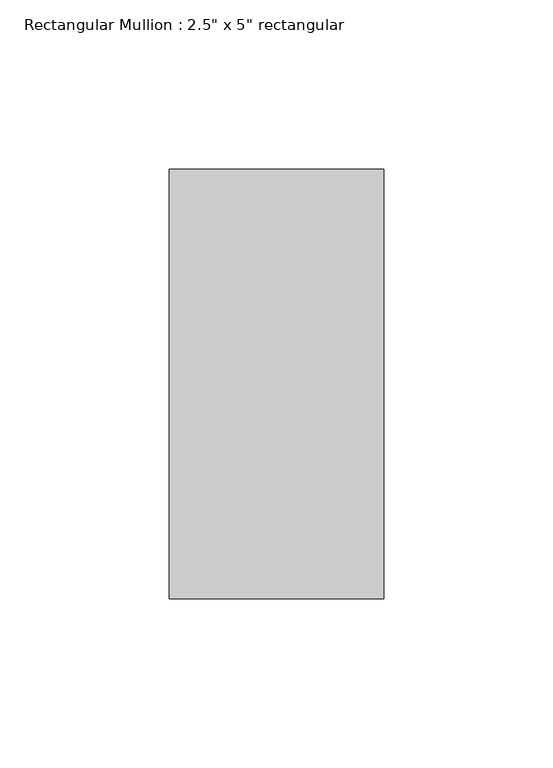
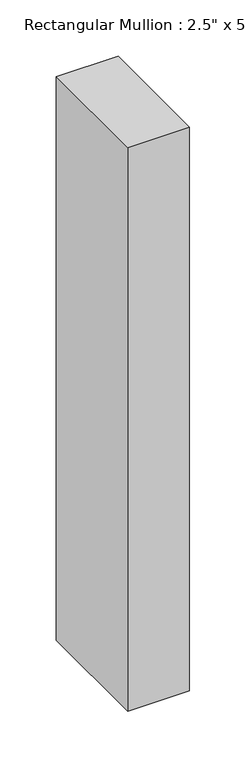
"""IFC4 building model written with IfcOpenShell, lengths in millimetres: member geometry."""

from ifc_helpers import new_model, si_unit, frame, origin, place, context, project, spatial, polyline, outline, extrude, source, transform, mapped, element, save


def member_cfc9b631(model_context):
    return source(origin(), model_context, "Body", "SweptSolid", [
        extrude(outline(polyline([(31.75, 63.5), (31.75, -63.5), (-31.75, -63.5), (-31.75, 63.5), (31.75, 63.5)])), frame((0.0, 0.0, -612.7937999), z_axis=(0.0, 0.0, 1.0), x_axis=(1.0, 0.0, 0.0)), (0.0, 0.0, 1.0), 612.7937999),
    ])


if __name__ == "__main__":
    model = new_model("IFC4")
    model_context = context("Model", 3, world=origin())
    ifc_project = project(units=[si_unit("LENGTHUNIT", "METRE", prefix="MILLI")], contexts=[model_context])
    site = spatial("IfcSite", under=ifc_project)
    building = spatial("IfcBuilding", under=site)
    placement = place(None, origin())
    member_shape = member_cfc9b631(model_context)
    element("IfcMember", 1, ObjectType="Rectangular Mullion : 2.5\" x 5\" rectangular", at=placement, inside=building, context=model_context, shape_type="MappedRepresentation", body=[
        mapped(member_shape, transform((0.0, 0.0, 0.0), x_axis=(1.0, 0.0, 0.0), y_axis=(0.0, 1.0, 0.0), z_axis=(0.0, 0.0, 1.0))),
    ])
    save(model, "model.ifc")

# Revit data of these elements
# Type "Rectangular Mullion : 2.5\" x 5\" rectangular"
#   built-in parameter 1007304 = 0.416667 (stored number, unit not read)
#   built-in parameter 1007301 = 0.104167 (stored number, unit not read)
#   built-in parameter 1007300 = 0.104167 (stored number, unit not read)
# Element 1 (IfcMember, "Rectangular Mullion : 2.5\" x 5\" rectangular")
#   Materials on its faces: "Aluminum"
# Materials
#   "Aluminum": class "Metal", colour RGB 247 247 247, transparency 0, Description = "Aluminum 6061", Cost = 0
